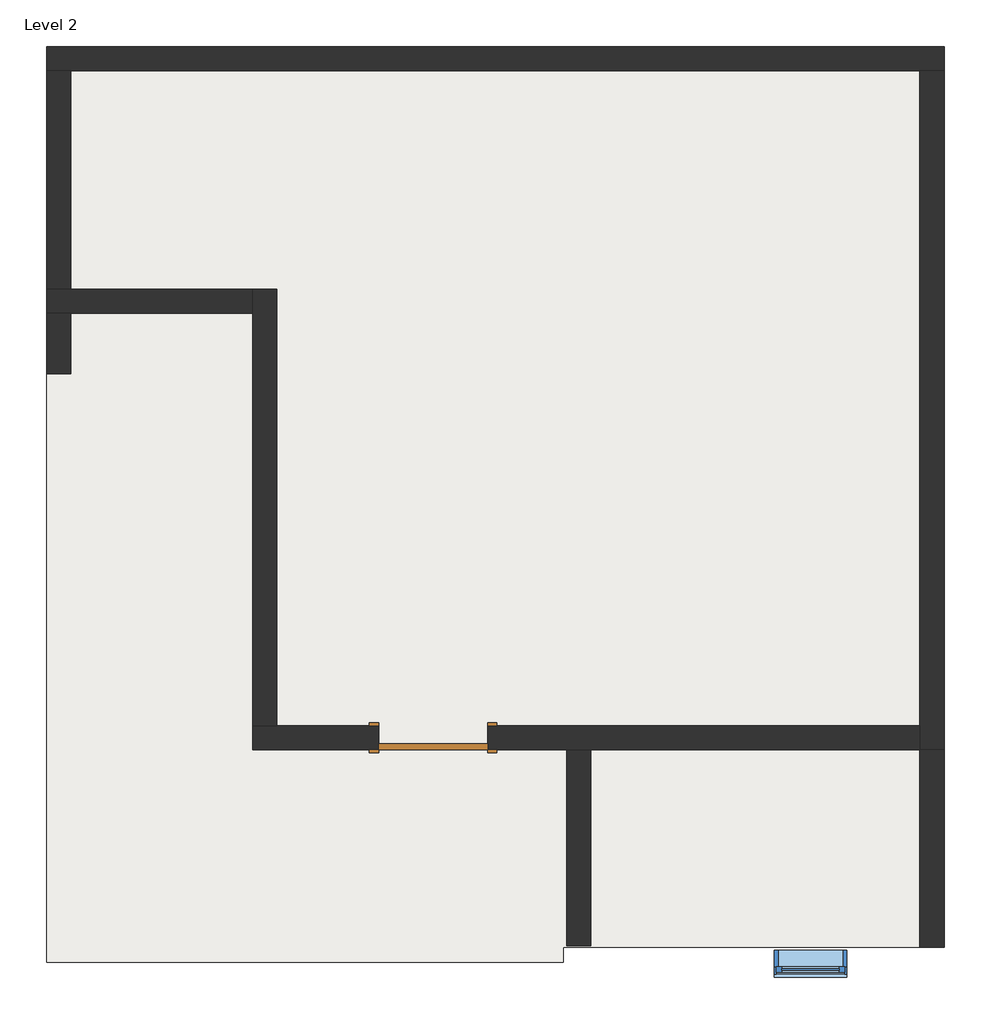
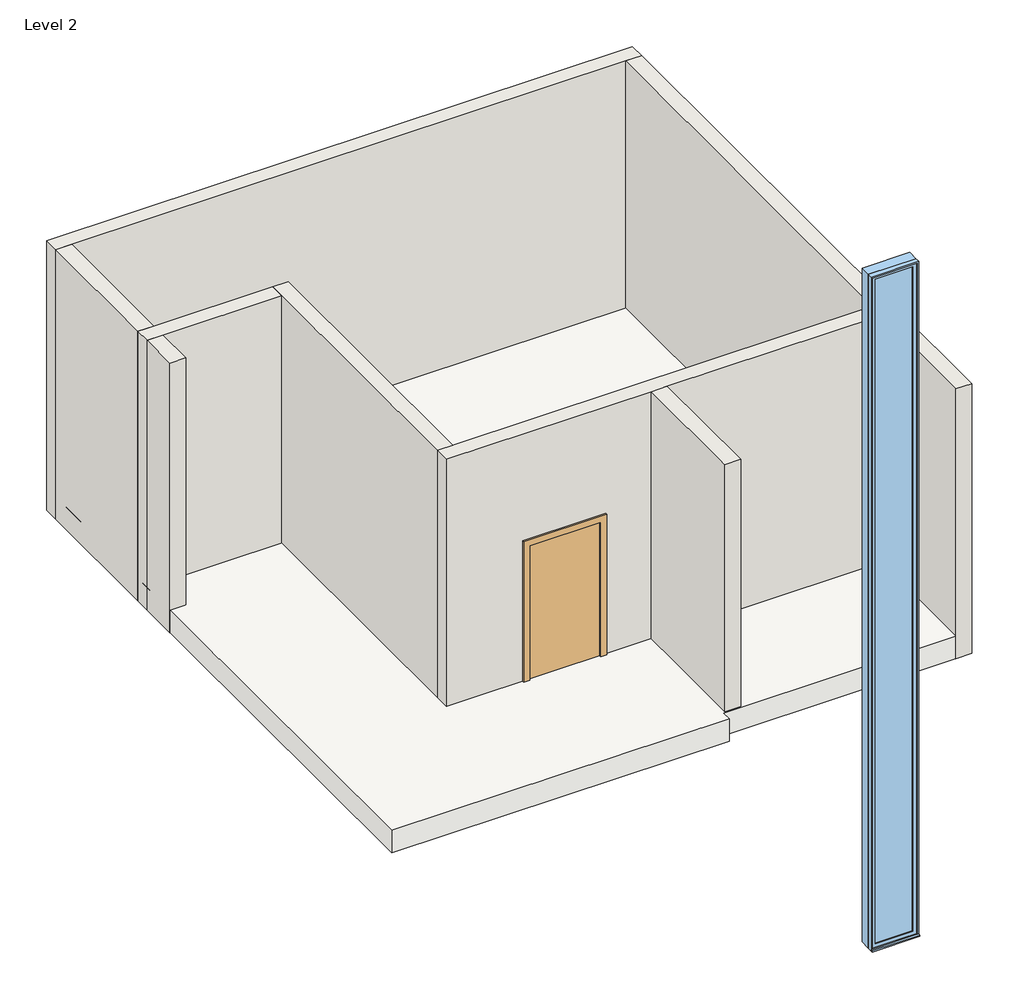
# One storey, incomplete: 9 walls, 1 door, 1 roof, 1 window.
"""IFC4 building model written with IfcOpenShell, lengths in millimetres."""

from ifc_helpers import new_model, si_unit, frame, origin, place, context, project, spatial, polyline, outline, extrude, faceted_brep, transform, mapped, element, save
from components import door_54dd4da4, window_44a3cfc2

model = new_model("IFC4")

# Units and contexts
model_context = context("Model", 3, world=origin())
ifc_project = project(units=[si_unit("LENGTHUNIT", "METRE", prefix="MILLI")], contexts=[model_context])

# Site, building, storey
site = spatial("IfcSite", under=ifc_project)
building = spatial("IfcBuilding", under=site)
storey = spatial("IfcBuildingStorey", under=building, Name="Level 2", Elevation=3657.6)

# Door
placement = place(None, origin())
door_shape = door_54dd4da4(model_context)
element("IfcDoor", 1, ObjectType="Single-Flush : 36\" x 84\"", at=placement, inside=storey, context=model_context, shape_type="MappedRepresentation", body=[
    mapped(door_shape, transform((-4477.6125658, 5951.9483979, 3657.6), x_axis=(-1.0, 0.0, 0.0), y_axis=(0.0, -1.0, 0.0), z_axis=(0.0, 0.0, 1.0))),
])

# Roof
element("IfcRoof", 2, ObjectType="Generic - 12\"", at=placement, inside=storey, context=model_context, shape_type="SweptSolid", body=[
    extrude(outline(polyline([(-7716.1125658, 11743.1483979), (-197.7125658, 11743.1483979), (-197.7125658, 4199.3483979), (-3385.4125658, 4199.3483979), (-3385.4125658, 4072.3483979), (-7716.1125658, 4072.3483979), (-7716.1125658, 11743.1483979)])), frame((0.0, 0.0, 3657.6), z_axis=(0.0, 0.0, 1.0), x_axis=(1.0, 0.0, 0.0)), (0.0, 0.0, 1.0), 304.8),
])

# Walls
element("IfcWall", 3, ObjectType="Generic - 8\"", at=placement, inside=storey, context=model_context, shape_type="Brep", body=[
    faceted_brep([(-7716.1125658, 11539.9483979, 3657.6), (-7512.9125658, 11539.9483979, 3657.6), (-400.9125658, 11539.9483979, 3657.6), (-197.7125658, 11539.9483979, 3657.6), (-197.7125658, 11539.9483979, 7315.2), (-400.9125658, 11539.9483979, 7315.2), (-7512.9125658, 11539.9483979, 7315.2), (-7716.1125658, 11539.9483979, 7315.2), (-7716.1125658, 11743.1483979, 3657.6), (-7716.1125658, 11743.1483979, 7315.2), (-197.7125658, 11743.1483979, 7315.2), (-197.7125658, 11743.1483979, 3657.6)], [[[0, 1, 2, 3, 4, 5, 6, 7]], [[8, 9, 10, 11]], [[3, 2, 1, 0, 8, 11]], [[7, 6, 5, 4, 10, 9]], [[4, 3, 11, 10]], [[0, 7, 9, 8]]]),
])
element("IfcWall", 4, ObjectType="Generic - 8\"", at=placement, inside=storey, context=model_context, shape_type="Brep", body=[
    faceted_brep([(-400.9125658, 11539.9483979, 3657.6), (-400.9125658, 6053.5483979, 3657.6), (-400.9125658, 5850.3483979, 3657.6), (-400.9125658, 5850.3483979, 7315.2), (-400.9125658, 6053.5483979, 7315.2), (-400.9125658, 11539.9483979, 7315.2), (-197.7125658, 11539.9483979, 3657.6), (-197.7125658, 11539.9483979, 7315.2), (-197.7125658, 5850.3483979, 7315.2), (-197.7125658, 5850.3483979, 3657.6)], [[[0, 1, 2, 3, 4, 5]], [[6, 7, 8, 9]], [[2, 1, 0, 6, 9]], [[5, 4, 3, 8, 7]], [[0, 5, 7, 6]], [[3, 2, 9, 8]]]),
])
element("IfcWall", 5, ObjectType="Generic - 8\"", at=placement, inside=storey, context=model_context, shape_type="Brep", body=[
    faceted_brep([(-4934.8125658, 6053.5483979, 5791.2), (-4934.8125658, 6053.5483979, 3657.6), (-5785.7125658, 6053.5483979, 3657.6), (-5988.9125658, 6053.5483979, 3657.6), (-5988.9125658, 6053.5483979, 7315.2), (-5785.7125658, 6053.5483979, 7315.2), (-400.9125658, 6053.5483979, 7315.2), (-400.9125658, 6053.5483979, 3657.6), (-4020.4125658, 6053.5483979, 3657.6), (-4020.4125658, 6053.5483979, 5791.2), (-5988.9125658, 5850.3483979, 3657.6), (-4934.8125658, 5850.3483979, 3657.6), (-4934.8125658, 5850.3483979, 5791.2), (-4020.4125658, 5850.3483979, 5791.2), (-4020.4125658, 5850.3483979, 3657.6), (-3360.0125658, 5850.3483979, 3657.6), (-3156.8125658, 5850.3483979, 3657.6), (-400.9125658, 5850.3483979, 3657.6), (-400.9125658, 5850.3483979, 7315.2), (-3156.8125658, 5850.3483979, 7315.2), (-3360.0125658, 5850.3483979, 7315.2), (-5988.9125658, 5850.3483979, 7315.2)], [[[0, 1, 2, 3, 4, 5, 6, 7, 8, 9]], [[10, 11, 12, 13, 14, 15, 16, 17, 18, 19, 20, 21]], [[8, 7, 17, 16, 15, 14]], [[3, 2, 1, 11, 10]], [[6, 5, 4, 21, 20, 19, 18]], [[7, 6, 18, 17]], [[4, 3, 10, 21]], [[12, 11, 1, 0]], [[13, 12, 0, 9]], [[14, 13, 9, 8]]]),
])
element("IfcWall", 6, ObjectType="Generic - 8\"", at=placement, inside=storey, context=model_context, shape_type="Brep", body=[
    faceted_brep([(-5785.7125658, 6053.5483979, 3657.6), (-5785.7125658, 9711.1483979, 3657.6), (-5785.7125658, 9711.1483979, 7315.2), (-5785.7125658, 6053.5483979, 7315.2), (-5988.9125658, 6053.5483979, 3657.6), (-5988.9125658, 6053.5483979, 7315.2), (-5988.9125658, 9507.9483979, 7315.2), (-5988.9125658, 9711.1483979, 7315.2), (-5988.9125658, 9711.1483979, 3657.6), (-5988.9125658, 9507.9483979, 3657.6)], [[[0, 1, 2, 3]], [[4, 5, 6, 7, 8, 9]], [[1, 0, 4, 9, 8]], [[3, 2, 7, 6, 5]], [[0, 3, 5, 4]], [[2, 1, 8, 7]]]),
])
element("IfcWall", 7, ObjectType="Generic - 8\"", at=placement, inside=storey, context=model_context, shape_type="Brep", body=[
    faceted_brep([(-5988.9125658, 9711.1483979, 3657.6), (-7512.9125658, 9711.1483979, 3657.6), (-7716.1125658, 9711.1483979, 3657.6), (-7716.1125658, 9711.1483979, 7315.2), (-7512.9125658, 9711.1483979, 7315.2), (-5988.9125658, 9711.1483979, 7315.2), (-5988.9125658, 9507.9483979, 3657.6), (-5988.9125658, 9507.9483979, 7315.2), (-7512.9125658, 9507.9483979, 7315.2), (-7716.1125658, 9507.9483979, 7315.2), (-7716.1125658, 9507.9483979, 3657.6), (-7512.9125658, 9507.9483979, 3657.6)], [[[0, 1, 2, 3, 4, 5]], [[6, 7, 8, 9, 10, 11]], [[2, 1, 0, 6, 11, 10]], [[5, 4, 3, 9, 8, 7]], [[0, 5, 7, 6]], [[3, 2, 10, 9]]]),
])
element("IfcWall", 8, ObjectType="Generic - 8\"", at=placement, inside=storey, context=model_context, shape_type="SweptSolid", body=[
    extrude(outline(polyline([(-7512.9125658, 11539.9483979), (-7512.9125658, 9711.1483979), (-7716.1125658, 9711.1483979), (-7716.1125658, 11539.9483979), (-7512.9125658, 11539.9483979)])), frame((0.0, 0.0, 3657.6), z_axis=(0.0, 0.0, 1.0), x_axis=(1.0, 0.0, 0.0)), (0.0, 0.0, 1.0), 3657.6),
])
element("IfcWall", 9, ObjectType="Generic - 8\"", at=placement, inside=storey, context=model_context, shape_type="SweptSolid", body=[
    extrude(outline(polyline([(-3360.0125658, 4212.0483979), (-3360.0125658, 5850.3483979), (-3156.8125658, 5850.3483979), (-3156.8125658, 4212.0483979), (-3360.0125658, 4212.0483979)])), frame((0.0, 0.0, 3657.6), z_axis=(0.0, 0.0, 1.0), x_axis=(1.0, 0.0, 0.0)), (0.0, 0.0, 1.0), 3657.6),
])
element("IfcWall", 10, ObjectType="Generic - 8\"", at=placement, inside=storey, context=model_context, shape_type="SweptSolid", body=[
    extrude(outline(polyline([(-400.9125658, 4199.3483979), (-400.9125658, 5850.3483979), (-197.7125658, 5850.3483979), (-197.7125658, 4199.3483979), (-400.9125658, 4199.3483979)])), frame((0.0, 0.0, 3657.6), z_axis=(0.0, 0.0, 1.0), x_axis=(1.0, 0.0, 0.0)), (0.0, 0.0, 1.0), 3657.6),
])
element("IfcWall", 11, ObjectType="Generic - 8\"", at=placement, inside=storey, context=model_context, shape_type="SweptSolid", body=[
    extrude(outline(polyline([(-7716.1125658, 8999.9483979), (-7716.1125658, 9507.9483979), (-7512.9125658, 9507.9483979), (-7512.9125658, 8999.9483979), (-7716.1125658, 8999.9483979)])), frame((0.0, 0.0, 3657.6), z_axis=(0.0, 0.0, 1.0), x_axis=(1.0, 0.0, 0.0)), (0.0, 0.0, 1.0), 3657.6),
])

# Window
window_shape = window_44a3cfc2(model_context)
element("IfcWindow", 12, ObjectType="Instance - Fixed : 24\" x 360\"", at=placement, inside=storey, context=model_context, shape_type="MappedRepresentation", body=[
    mapped(window_shape, transform((-1353.4125658, 4072.3483979, -5842.0), x_axis=(-1.0, 0.0, 0.0), y_axis=(0.0, -1.0, 0.0), z_axis=(0.0, 0.0, 1.0))),
])

save(model, "model.ifc")

# Revit data of these elements
# Type "Single-Flush : 36\" x 84\""
#   Type Mark = "1"
#   Construction Type Id = "MDOOR"
#   Assembly Code = "C1020"
#   Analytic Construction = "Metal"
#   Thickness = 0' - 2"
#   Heat Transfer Coefficient (U) = 0.651978 BTU/(h·ft²·°F)
#   Height = 7' - 0"
#   Trim Projection Ext = 0' - 1"
#   Trim Projection Int = 0' - 1"
#   Trim Width = 0' - 3"
#   Width = 3' - 0"
#   Define Thermal Properties by = 1
#   Door Material = Door - Panel
#   Frame Material = Door - Frame
#   Visual Light Transmittance = 0
#   Solar Heat Gain Coefficient = 0
#   Function = (empty or 0)
#   Wall Closure = (empty or 0)
# Type "Generic - 12\""
#   Assembly Code = "B1020"
#   Layers, outside or top first: 1' - 0" no material (function 1)
# Type "Generic - 8\""
#   Assembly Code = "B2010"
#   Layers, outside or top first: 0' - 8" no material (function 1)
# Type "Instance - Fixed : 24\" x 360\""
#   Type Mark = "10"
#   Construction Type Id = "GSP4R"
#   Assembly Code = "B2020100"
#   Analytic Construction = "1/8 in Pilkington single glazing"
#   Visual Light Transmittance = 0.9
#   Thermal Resistance (R) = 0.8466 (h·ft²·°F)/BTU
#   Solar Heat Gain Coefficient = 0.86
#   Heat Transfer Coefficient (U) = 1.1812 BTU/(h·ft²·°F)
#   Height [instance default] = 4' - 0"
#   Default Sill Height = 20' - 0"
#   Width [instance default] = 2' - 0"
#   Window Inset = 0' - 0 3/4"
#   Define Thermal Properties by = 1
#   Glass Pane Material = Glass
#   Sash Material = Default Roof
#   Wall Closure = (empty or 0)
# Element 1 (IfcDoor, "Single-Flush : 36\" x 84\"")
#   Phase Created = New Construction
#   Materials on its faces: "Door - Frame", "Door - Panel"
# Element 2 (IfcRoof, "Generic - 12\"")
#   built-in parameter 1001705 = 13 (stored number, unit not read)
#   built-in parameter 1001710 = 33615
#   Phase Created = New Construction
#   Materials on its faces: "Default Roof"
# Elements 3, 4, 5, 6, 7, 8, 9, 10, 11 (IfcWall, "Generic - 8\"")
#   Top Offset = 0' - 0"
#   Base Offset = 0' - 0"
#   Unconnected Height = 12' - 0"
#   wall height = 12' - 0"
#   Phase Created = New Construction
#   Base Constraint = Level 2
#   Materials on its faces: "Default Wall"
# Element 12 (IfcWindow, "Instance - Fixed : 24\" x 360\"")
#   Mark = "1"
#   Width = 2' - 0"
#   Height = 30' - 0"
#   Phase Created = New Construction
#   Materials on its faces: "Default Roof", "Glass"
# Materials
#   "Door - Panel": class "Wood", colour RGB 210 159 95, transparency 0
#   "Door - Frame": colour RGB 118 70 51, transparency 0
#   "Glass": class "Glass", colour RGB 0 128 192, transparency 0.75, Description = "Soda Lime Glass", Cost = 0
#   "Default Roof": colour RGB 88 101 114, transparency 0
#   "Default Wall": colour RGB 128 128 128, transparency 0
